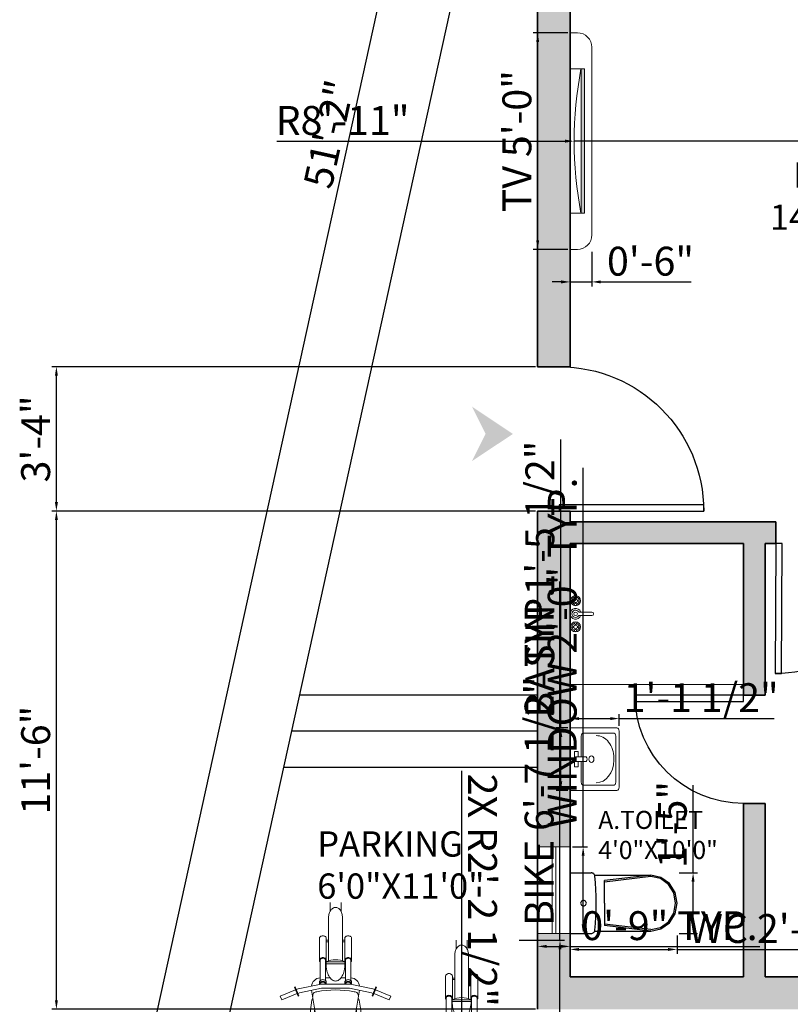
# Model space of a CAD drawing. Units: inches. Extents: x 2642 to 4124, y 1227 to 1973.
# Tile 2 of 7: x 3343 to 3556, y 1372 to 1645. Entities that reach past the tile are written whole.
import ezdxf

# ---------------------------------------------------------------- set-up
doc = ezdxf.new("R2010")
doc.units = ezdxf.units.IN
for name, color, linetype, lineweight in [('A-ANNO-DIMS', 2, 'Continuous', 18), ('A-ANNO-SYMB', 1, 'Continuous', 18), ('A-AREA-IDEN', 7, 'Continuous', 18), ('A-DOOR', 3, 'Continuous', 25), ('A-EQPM', 8, 'Continuous', 18), ('A-FLOR-STRS', 7, 'Continuous', 25), ('A-WALL', 7, 'Continuous', 35), ('A-WALL-PATT', 7, 'Continuous', 13), ('C-PRKG-VEHI', 8, 'Continuous', 18), ('C-PROP', 7, 'Continuous', 25), ('window', 4, 'Continuous', 18), ('Сантехника', 9, 'Continuous', 18)]:
    doc.layers.add(name, color=color, linetype=linetype, lineweight=lineweight)
doc.layers.add('SANTEH', color=7, linetype='Continuous')
doc.styles.get("Standard").update_dxf_attribs({"font": 'arial.ttf'})
doc.dimstyles.new('ISO-25', dxfattribs={"dimtxt": 8, "dimasz": 2.5, "dimexe": 1.25, "dimexo": 0.625, "dimtad": 1, "dimdec": 0, "dimlunit": 3, "dimtxsty": 'Standard', "dimcen": 2.5, "dimadec": 0, "dimazin": 0, "dimtfac": 1, "dimtdec": 0, "dimtmove": 0, "dimatfit": 3, "dimfxl": 1, "dimarcsym": 0})

# ---------------------------------------------------------------- blocks, each defined once
blk = doc.blocks.new('*D4')
at = {"layer": 'A-ANNO-DIMS', "color": 0, "lineweight": -2, "transparency": 16777216}
for p, q in [((3518.61, 1907.92), (3498.8, 1912.28)), ((3368.56, 1314.45), (3499.49, 1909.57)), ((3386.61, 1307.92), (3366.8, 1312.28))]:
    blk.add_line(p, q, dxfattribs=at)
at = {"layer": 'A-ANNO-DIMS', "color": 0, "transparency": 16777216}
for points in [[(3499.08, 1909.65), (3499.89, 1909.48), (3500.02, 1912.01)], [(3368.15, 1314.54), (3368.97, 1314.36), (3368.02, 1312.01)]]:
    blk.add_solid(points, dxfattribs=at)
at = {"layer": 'Defpoints', "color": 0, "transparency": 16777216}
for p in [(3500.02, 1912.01), (3519.22, 1907.78), (3387.22, 1307.78)]:
    blk.add_point(p, dxfattribs=at)
at = {"layer": 'A-ANNO-DIMS', "color": 0, "transparency": 16777216, "insert": (3429.42, 1613.02), "char_height": 8, "attachment_point": 5, "rotation": 77.5926}
blk.add_mtext('51\'-2"', dxfattribs=at)
blk = doc.blocks.new('*U11')
for p, q in [((0, 0), (0, -6)), ((30, 0), (30, -6))]:
    blk.add_line(p, q)
blk.add_lwpolyline([(0, 0), (0, 30), (1.75, 30), (1.75, 0)], close=True)
blk.add_arc((0, 0), 30, 0, 90)
blk = doc.blocks.new('*U10')
for p, q in [((0, 0), (0, -6)), ((36, 0), (36, -6))]:
    blk.add_line(p, q)
blk.add_lwpolyline([(0, 0), (0, 36), (1.75, 36), (1.75, 0)], close=True)
blk.add_arc((0, 0), 36, 0, 90)
blk = doc.blocks.new('*U13')
for p, q in [((0, 0), (0, -6)), ((40, 0), (40, -6))]:
    blk.add_line(p, q)
blk.add_lwpolyline([(0, 0), (0, 40), (1.75, 40), (1.75, 0)], close=True)
blk.add_arc((0, 0), 40, 0, 90)
blk = doc.blocks.new('TV 1')
at = {"transparency": 33554687}
h = blk.add_hatch(color=256, dxfattribs=at)
h.dxf.hatch_style = 1
h.paths.add_polyline_path([(3528.27, 1618.89), (3528.27, 1617.89), (3568.27, 1617.89), (3568.27, 1618.89)])
for p, q in [((3574.27, 1620.89), (3522.27, 1620.89)), ((3528.27, 1614.89), (3528.27, 1618.89)), ((3528.27, 1618.89), (3568.27, 1618.89)), ((3528.27, 1617.89), (3568.27, 1617.89)), ((3568.27, 1614.89), (3568.27, 1618.89)), ((3518.27, 1614.89), (3518.27, 1616.89)), ((3578.27, 1614.89), (3578.27, 1616.89)), ((3518.27, 1614.89), (3578.27, 1614.89))]:
    blk.add_line(p, q)
for centre, radius, start, end in [((3522.27, 1616.89), 4, 90, 180), ((3574.27, 1616.89), 4, 0, 90), ((3548.27, 1722.92), 106.92, 259.2189, 280.7811)]:
    blk.add_arc(centre, radius, start, end)
blk = doc.blocks.new('Rac7')
at = {"color": 0}
for p, q in [((-39473.6, -23808.4), (-38988.3, -23808.4)), ((-39500.6, -24232.1), (-39500.6, -23829.6)), ((-39456.5, -23859.1), (-39456.5, -24114.9)), ((-39032.4, -23838), (-39429.6, -23838)), ((-39221.1, -23854.9), (-39240.8, -23854.9)), ((-39005.4, -24114.9), (-39005.4, -23859.1)), ((-39005.4, -23859.1), (-39005.4, -23859.1)), ((-38961.3, -23829.6), (-38961.3, -24232.1)), ((-39429.6, -24136.1), (-39252.5, -24136.1)), ((-39252.5, -24185.9), (-39252.5, -24093.6)), ((-39209.4, -24185.9), (-39209.4, -24093.6)), ((-39209.4, -24136.1), (-39032.4, -24136.1)), ((-38961.3, -24232.1), (-39500.6, -24232.1)), ((-39297, -24164), (-39252.5, -24164)), ((-39297, -24193.5), (-39297, -24164)), ((-39164.9, -24193.5), (-39297, -24193.5)), ((-39252.5, -24185.9), (-39209.4, -24185.9)), ((-39209.4, -24164), (-39164.9, -24164)), ((-39164.9, -24164), (-39164.9, -24193.5))]:
    blk.add_line(p, q, dxfattribs=at)
at = {"color": 0, "extrusion": (0, 0, -1)}
for centre, major_axis, start_param, end_param in [((-39473.6, -23829.6), (-27, 0), 0, 1.570796), ((-38988.3, -23829.6), (-27, 0), 1.570796, 3.141593), ((-39429.6, -23859.1), (-27, 0), 0, 1.570796), ((-39240.8, -24007.4), (-194.1, 0), 0, 1.570796), ((-39221.1, -24007.4), (-194.1, 0), 1.570796, 3.141593), ((-39032.4, -23859.1), (-27, 0), 1.570796, 3.141593), ((-39429.6, -24114.9), (-27, 0), -1.570796, 0), ((-39231, -24104), (-25.3, 0), 0.552816, 2.588777), ((-39032.4, -24114.9), (-27, 0), -3.141593, -1.570796)]:
    blk.add_ellipse(centre, major_axis=major_axis, ratio=0.785714, start_param=start_param, end_param=end_param, dxfattribs=at)
blk.add_ellipse((-39231, -24048), major_axis=(-27.9, 0), ratio=0.785714, dxfattribs=at)
blk = doc.blocks.new('Faucet - Bathroom top')
for p, q in [((-4.107, 0.125), (-4.375, 0.125)), ((-3.75, 0.4788), (-3.75, 0.75)), ((-3.5, 0.482), (-3.5, 0.75)), ((-3.1461, 0.125), (-2.875, 0.125)), ((3.143, 0.125), (2.875, 0.125)), ((3.5, 0.4788), (3.5, 0.75)), ((3.75, 0.482), (3.75, 0.75)), ((4.1039, 0.125), (4.375, 0.125)), ((-4.1039, -0.125), (-4.375, -0.125)), ((-3.75, -0.4821), (-3.75, -0.75)), ((-3.5, -0.4789), (-3.5, -0.75)), ((-3.143, -0.125), (-2.875, -0.125)), ((-0.5, -0.8639), (-0.5, -4.5)), ((0.5, -4.5), (0.5, -0.8631)), ((3.1461, -0.125), (2.875, -0.125)), ((3.5, -0.4821), (3.5, -0.75)), ((3.75, -0.4789), (3.75, -0.75)), ((4.107, -0.125), (4.375, -0.125))]:
    blk.add_line(p, q)
for centre, radius in [((-3.625, 0), 1.375), ((-4.625, 0), 0.2795), ((-3.625, 0), 0.5), ((-3.625, 1), 0.2795), ((-2.625, 0), 0.2795), ((0, 0), 0.5), ((3.625, 0), 1.375), ((2.625, 0), 0.2795), ((3.625, 0), 0.5), ((3.625, 1), 0.2795), ((4.625, 0), 0.2795), ((-3.625, -1), 0.2795), ((3.625, -1), 0.2795)]:
    blk.add_circle(centre, radius)
for centre, radius, start, end in [((-3.625, 0), 1, 105.2407, 164.2093), ((-3.625, 0), 1, 16.44125, 74.07887), ((0, 0), 1.5, 289.6514, 250.3603), ((0, 0), 1, 300.3431, 239.7554), ((3.625, 0), 1, 106.12, 164.0884), ((3.625, 0), 1, 16.23422, 73.90469), ((-3.625, 0), 1, 196.2342, 253.9047), ((-3.625, 0), 1, 286.12, 344.0884), ((3.625, 0), 1, 196.4413, 254.0789), ((3.625, 0), 1, 285.2407, 344.2093), ((0, -4.5), 0.5, 180, 0)]:
    blk.add_arc(centre, radius, start, end)
blk = doc.blocks.new('WC 2 Symb_109')
at = {"layer": 'SANTEH'}
for p, q in [((0, 0), (0, 380)), ((0, 380), (132.4, 380)), ((153.6, 364.9), (506.8, 364.9)), ((506.3, 364.9), (215.7, 330.9)), ((506.3, 356), (215.7, 322)), ((215.7, 190), (215.7, 330.9)), ((215.7, 190), (215.7, 49.1)), ((153.8, 15.1), (506.8, 15.1)), ((506.3, 24), (215.7, 58)), ((506.3, 15.1), (215.7, 49.1)), ((0, 0), (132.4, 0))]:
    blk.add_line(p, q, dxfattribs=at)
for points in [[(154.6, 360.1), (153.9, 364.1), (152.3, 367.9), (150.2, 371.3), (147.4, 374.3), (144.1, 376.7), (140.5, 378.5), (136.5, 379.6), (132.4, 380)], [(154.6, 19.7), (158.6, 62.1), (161.4, 104.7), (163.1, 147.3), (163.7, 189.9), (163.1, 232.5), (161.4, 275.1), (158.6, 317.7), (154.6, 360.1)], [(506.3, 24), (565.5, 36.6), (615.7, 72.6), (649.2, 126.5), (661, 190), (649.2, 253.5), (615.7, 307.4), (565.5, 343.4), (506.3, 356)], [(506.8, 15.1), (569.2, 28.4), (622.2, 66.3), (657.6, 123.1), (670, 190), (657.6, 256.9), (622.2, 313.7), (569.2, 351.6), (506.8, 364.9)], [(132.4, 0), (136.5, 0.4), (140.4, 1.5), (144.1, 3.2), (147.3, 5.6), (150.1, 8.6), (152.3, 12), (153.8, 15.7), (154.6, 19.7)]]:
    blk.add_lwpolyline(points, dxfattribs=at)
blk.add_lwpolyline([(83.6, 208.5), (70.4, 203.1), (64.9, 190), (70.4, 176.9), (83.6, 171.5), (96.8, 176.9), (102.2, 190), (96.8, 203.1)], close=True, dxfattribs=at)
blk = doc.blocks.new('BIKE')
for p, q in [((34846.04, 15170.34), (34846.04, 15168.87)), ((34847.86, 15170.34), (34847.86, 15168.87)), ((34845.81, 15167.86), (34845.81, 15160.7)), ((34845.81, 15167.86), (34845.81, 15160.7)), ((34848.09, 15167.86), (34848.09, 15160.7)), ((34844.29, 15164.4), (34844.29, 15160.81)), ((34845.43, 15164.4), (34845.43, 15160.81)), ((34845.43, 15164.1), (34845.81, 15164.1)), ((34845.43, 15163.85), (34845.81, 15163.85)), ((34848.47, 15164.1), (34848.09, 15164.1)), ((34848.47, 15163.85), (34848.09, 15163.85)), ((34848.47, 15164.4), (34848.47, 15160.81)), ((34849.61, 15164.4), (34849.61, 15160.81)), ((34844.41, 15160.81), (34844.41, 15157.43)), ((34845.32, 15160.81), (34845.32, 15157.43)), ((34848.51, 15160.53), (34845.39, 15160.53)), ((34845.39, 15160.23), (34845.39, 15160.53)), ((34845.39, 15160.23), (34845.39, 15160.53)), ((34848.51, 15160.23), (34845.39, 15160.23)), ((34848.51, 15160.23), (34848.51, 15160.53)), ((34848.58, 15160.81), (34848.58, 15157.43)), ((34849.5, 15160.81), (34849.5, 15157.43)), ((34840.8, 15156.11), (34844.56, 15156.88)), ((34844.29, 15156.87), (34844.29, 15157.17)), ((34844.41, 15156.87), (34844.41, 15156.85)), ((34844.56, 15156.88), (34846.95, 15156.88)), ((34845.32, 15157.92), (34846.04, 15157.92)), ((34845.43, 15156.87), (34845.43, 15157.17)), ((34849.34, 15156.88), (34846.95, 15156.88)), ((34848.58, 15157.92), (34847.87, 15157.92)), ((34848.47, 15156.87), (34848.47, 15157.17)), ((34853.1, 15156.11), (34849.34, 15156.88)), ((34849.5, 15156.87), (34849.5, 15156.85)), ((34849.61, 15156.87), (34849.61, 15157.17)), ((34837.84, 15154.89), (34840.37, 15155.93)), ((34838.1, 15154.26), (34840.63, 15155.3)), ((34840.19, 15156.35), (34840.3, 15156.39)), ((34840.19, 15156.35), (34840.8, 15154.88)), ((34840.3, 15156.39), (34840.9, 15154.92)), ((34840.47, 15155.97), (34840.8, 15156.11)), ((34840.73, 15155.34), (34841, 15155.45)), ((34841, 15155.45), (34844.63, 15156.2)), ((34844.86, 15144.72), (34843.01, 15155.87)), ((34844.63, 15156.2), (34846.95, 15156.2)), ((34849.27, 15156.2), (34846.95, 15156.2)), ((34849.05, 15144.72), (34850.89, 15155.87)), ((34852.9, 15155.45), (34849.27, 15156.2)), ((34853.17, 15155.34), (34852.9, 15155.45)), ((34853.6, 15156.39), (34853, 15154.92)), ((34853.71, 15156.35), (34853.1, 15154.88)), ((34853.43, 15155.97), (34853.1, 15156.11)), ((34855.81, 15154.26), (34853.28, 15155.3)), ((34856.07, 15154.89), (34853.54, 15155.93)), ((34853.71, 15156.35), (34853.6, 15156.39)), ((34837.84, 15154.89), (34838.1, 15154.26)), ((34840.8, 15154.88), (34840.9, 15154.92)), ((34842.8, 15152.59), (34843.06, 15154.2)), ((34843.06, 15154.2), (34843.22, 15154.58)), ((34850.84, 15154.2), (34850.68, 15154.58)), ((34851.1, 15152.59), (34850.84, 15154.2)), ((34853.1, 15154.88), (34853, 15154.92)), ((34856.07, 15154.89), (34855.81, 15154.26)), ((34842.7, 15150.31), (34842.8, 15152.59)), ((34843.33, 15151.09), (34843.52, 15152.8)), ((34850.57, 15151.09), (34850.38, 15152.8)), ((34851.2, 15150.31), (34851.1, 15152.59)), ((34840.97, 15150.31), (34843.3, 15150.31)), ((34840.97, 15149.81), (34840.97, 15150.31)), ((34843.23, 15147.75), (34843.33, 15151.09)), ((34850.67, 15147.75), (34850.57, 15151.09)), ((34852.93, 15150.31), (34850.6, 15150.31)), ((34852.93, 15149.81), (34852.93, 15150.31)), ((34843.29, 15149.81), (34840.97, 15149.81)), ((34842.7, 15144.87), (34842.7, 15149.81)), ((34850.61, 15149.81), (34852.93, 15149.81)), ((34851.2, 15144.87), (34851.2, 15149.81)), ((34843.23, 15144.15), (34843.23, 15147.75)), ((34850.67, 15144.15), (34850.67, 15147.75)), ((34842.7, 15144.87), (34842.25, 15142.19)), ((34842.7, 15144.87), (34843.23, 15144.87)), ((34847.85, 15144.64), (34846.06, 15144.64)), ((34851.2, 15144.87), (34850.67, 15144.87)), ((34851.2, 15144.87), (34851.65, 15142.19)), ((34842.25, 15142.19), (34844.07, 15142.19)), ((34842.25, 15137.82), (34842.25, 15142.19)), ((34844.46, 15143.56), (34843.6, 15128.2)), ((34843.85, 15143.46), (34844.07, 15142.19)), ((34843.91, 15143.46), (34844.46, 15143.46)), ((34844.07, 15137.82), (34844.07, 15142.19)), ((34849.44, 15143.56), (34850.3, 15128.2)), ((34849.99, 15143.46), (34849.44, 15143.46)), ((34850.05, 15143.46), (34849.83, 15142.19)), ((34851.65, 15142.19), (34849.83, 15142.19)), ((34849.83, 15137.82), (34849.83, 15142.19)), ((34851.65, 15137.82), (34851.65, 15142.19)), ((34841.79, 15137.82), (34844.14, 15137.82)), ((34841.79, 15137.33), (34841.79, 15137.82)), ((34844.11, 15137.33), (34841.79, 15137.33)), ((34842.25, 15127.57), (34842.25, 15137.33)), ((34844.07, 15136.55), (34844.07, 15137.33)), ((34852.11, 15137.82), (34849.76, 15137.82)), ((34849.79, 15137.33), (34852.11, 15137.33)), ((34849.83, 15136.55), (34849.83, 15137.33)), ((34851.65, 15127.57), (34851.65, 15137.33)), ((34852.11, 15137.33), (34852.11, 15137.82)), ((34842.25, 15127.57), (34843.75, 15127.57)), ((34842.25, 15127.57), (34842.48, 15126.27)), ((34851.65, 15127.57), (34850.15, 15127.57)), ((34851.65, 15127.57), (34851.43, 15126.27)), ((34842.48, 15126.27), (34843.84, 15126.27)), ((34844.02, 15127.25), (34843.84, 15126.27)), ((34849.16, 15126.99), (34844.74, 15126.99)), ((34845.47, 15126.99), (34845.47, 15126.88)), ((34845.81, 15126.99), (34845.81, 15126.88)), ((34845.81, 15126.29), (34845.81, 15124.03)), ((34847.75, 15126.54), (34846.15, 15126.54)), ((34847.75, 15126.2), (34846.15, 15126.2)), ((34848.09, 15126.99), (34848.09, 15126.88)), ((34848.09, 15126.29), (34848.09, 15124.03)), ((34848.43, 15126.99), (34848.43, 15126.88)), ((34849.89, 15127.25), (34850.06, 15126.27)), ((34851.43, 15126.27), (34850.06, 15126.27)), ((34846.29, 15123.82), (34846.29, 15124.66)), ((34846.29, 15124.66), (34847.61, 15124.66)), ((34846.29, 15124.55), (34847.61, 15124.55)), ((34847.61, 15124.66), (34847.61, 15123.82)), ((34847.61, 15123.82), (34846.29, 15123.82))]:
    blk.add_line(p, q)
for points in [[(34845.81, 15167.86, -0.068977), (34845.9, 15168.53, -0.081012), (34846.15, 15169.05, -0.107014), (34846.54, 15169.42, -0.137239), (34846.95, 15169.53, -0.137239), (34847.36, 15169.42, -0.107014), (34847.76, 15169.05, -0.081012), (34848, 15168.53, -0.068977), (34848.09, 15167.86, -0.068977)], [(34845.43, 15164.4, 0.125099), (34845.39, 15164.56, 0.105827), (34845.27, 15164.71, 0.086577), (34845.09, 15164.8, 0.0766), (34844.86, 15164.84, 0.0766), (34844.64, 15164.8, 0.086577), (34844.46, 15164.71, 0.105827), (34844.33, 15164.56, 0.125099), (34844.29, 15164.4, 0.125099)], [(34848.47, 15164.4, -0.125099), (34848.51, 15164.56, -0.105827), (34848.64, 15164.71, -0.086577), (34848.82, 15164.8, -0.0766), (34849.04, 15164.84, -0.0766), (34849.26, 15164.8, -0.086577), (34849.44, 15164.71, -0.105827), (34849.57, 15164.56, -0.125099), (34849.61, 15164.4, -0.125099)], [(34845.32, 15160.55, 0.067261), (34845.39, 15160.65, 0.125099), (34845.43, 15160.81, 0.125099), (34845.39, 15160.97, 0.105827), (34845.27, 15161.12, 0.086577), (34845.09, 15161.21, 0.0766), (34844.86, 15161.25, 0.0766), (34844.64, 15161.21, 0.086577), (34844.46, 15161.12, 0.105827), (34844.33, 15160.97, 0.125099), (34844.29, 15160.81, 0.125099)], [(34844.29, 15160.81, 0.125099), (34844.33, 15160.65, 0.067261), (34844.41, 15160.55, 0.086577)], [(34845.32, 15160.81, 0.125099), (34845.29, 15160.92, 0.105827), (34845.2, 15161.03, 0.086577), (34845.05, 15161.1, 0.0766), (34844.86, 15161.13, 0.0766), (34844.67, 15161.1, 0.086577), (34844.53, 15161.03, 0.105827), (34844.43, 15160.92, 0.125099), (34844.41, 15160.81, 0.125099)], [(34846.95, 15157.37, -0.163989), (34846.41, 15157.55, -0.105862), (34845.85, 15158.21, -0.069323), (34845.52, 15159.08, -0.055531), (34845.39, 15160.23, -0.055531)], [(34848.51, 15160.23, -0.055531), (34848.38, 15159.08, -0.069323), (34848.06, 15158.21, -0.105862), (34847.49, 15157.55, -0.163989), (34846.95, 15157.37, -0.163989)], [(34848.58, 15160.55, -0.067261), (34848.51, 15160.65, -0.125099), (34848.47, 15160.81, -0.125099), (34848.51, 15160.97, -0.105827), (34848.64, 15161.12, -0.086577), (34848.82, 15161.21, -0.0766), (34849.04, 15161.25, -0.0766), (34849.26, 15161.21, -0.086577), (34849.44, 15161.12, -0.105827), (34849.57, 15160.97, -0.125099), (34849.61, 15160.81, -0.125099)], [(34848.58, 15160.81, -0.125099), (34848.61, 15160.92, -0.105827), (34848.71, 15161.03, -0.086577), (34848.85, 15161.1, -0.0766), (34849.04, 15161.13, -0.0766), (34849.23, 15161.1, -0.086577), (34849.37, 15161.03, -0.105827), (34849.47, 15160.92, -0.125099), (34849.5, 15160.81, -0.125099)], [(34849.61, 15160.81, -0.125099), (34849.57, 15160.65, -0.067261), (34849.5, 15160.55, -0.086577)], [(34845.43, 15157.17, 0.125099), (34845.39, 15157.33, 0.105827), (34845.27, 15157.48, 0.086577), (34845.09, 15157.57, 0.0766), (34844.86, 15157.6, 0.0766), (34844.64, 15157.57, 0.086577), (34844.46, 15157.48, 0.105827), (34844.33, 15157.33, 0.125099), (34844.29, 15157.17, 0.125099)], [(34845.43, 15156.88, 0.117252), (34845.39, 15157.03, 0.105827), (34845.27, 15157.18, 0.086577), (34845.09, 15157.27, 0.0766), (34844.86, 15157.31, 0.0766), (34844.64, 15157.27, 0.086577), (34844.46, 15157.18, 0.105827), (34844.33, 15157.03, 0.125099), (34844.29, 15156.87, 0.125099)], [(34844.29, 15156.87, 0.032819), (34844.3, 15156.83, 0.067261)], [(34845.32, 15156.88, 0.113202), (34845.29, 15156.98, 0.105827), (34845.2, 15157.09, 0.086577), (34845.05, 15157.16, 0.0766), (34844.86, 15157.19, 0.0766), (34844.67, 15157.16, 0.086577), (34844.53, 15157.09, 0.105827), (34844.43, 15156.98, 0.125099), (34844.41, 15156.87, 0.125099)], [(34848.47, 15157.17, -0.125099), (34848.51, 15157.33, -0.105827), (34848.64, 15157.48, -0.086577), (34848.82, 15157.57, -0.0766), (34849.04, 15157.6, -0.0766), (34849.26, 15157.57, -0.086577), (34849.44, 15157.48, -0.105827), (34849.57, 15157.33, -0.125099), (34849.61, 15157.17, -0.125099)], [(34848.47, 15156.88, -0.117252), (34848.51, 15157.03, -0.105827), (34848.64, 15157.18, -0.086577), (34848.82, 15157.27, -0.0766), (34849.04, 15157.31, -0.0766), (34849.26, 15157.27, -0.086577), (34849.44, 15157.18, -0.105827), (34849.57, 15157.03, -0.125099), (34849.61, 15156.87, -0.125099)], [(34848.58, 15156.88, -0.113202), (34848.61, 15156.98, -0.105827), (34848.71, 15157.09, -0.086577), (34848.85, 15157.16, -0.0766), (34849.04, 15157.19, -0.0766), (34849.23, 15157.16, -0.086577), (34849.37, 15157.09, -0.105827), (34849.47, 15156.98, -0.125099), (34849.5, 15156.87, -0.125099)], [(34849.61, 15156.87, -0.032819), (34849.61, 15156.83, -0.067261)]]:
    blk.add_lwpolyline(points, format="xyb")
for centre, radius, start, end in [((34846.95, 15157.24), 3.64, 64.5882, 115.4118), ((34844.55, 15156.32), 1.59, 95.2207, 171.678), ((34849.35, 15156.32), 1.59, 8.322, 84.7793), ((34843.86, 15154.92), 0.684, 90, 189.3898), ((34846.95, 15140.12), 15.79, 78.7129, 101.2871), ((34850.04, 15154.92), 0.684, 350.6102, 90), ((34843.91, 15144.15), 0.684, 180, 270), ((34846, 15143), 1.64, 88.1125, 159.9264), ((34845.53, 15144.83), 0.684, 189.3898, 226.4877), ((34847.9, 15143), 1.64, 20.0736, 91.8875), ((34848.37, 15144.83), 0.684, 313.5123, 350.6102), ((34849.99, 15144.15), 0.684, 270, 0), ((34844.74, 15128.13), 1.14, 176.7865, 270), ((34849.16, 15128.13), 1.14, 270, 3.2135), ((34846.15, 15126.88), 0.684, 180, 270), ((34846.15, 15126.88), 0.342, 180, 270), ((34847.75, 15126.88), 0.684, 270, 0), ((34847.75, 15126.88), 0.342, 270, 0), ((34846.95, 15124.03), 1.14, 180, 0)]:
    blk.add_arc(centre, radius, start, end)
blk = doc.blocks.new('WIN-24IN')
for p, q in [((0, 24), (9, 24)), ((4, 24), (4, 0)), ((5, 24), (5, 0)), ((0, 0), (9, 0))]:
    blk.add_line(p, q)
blk = doc.blocks.new('*D42')
at = {"layer": 'A-ANNO-DIMS', "color": 0, "lineweight": -2, "transparency": 16777216}
for p, q in [((3498.82, 1415.78), (3498.82, 1520.77)), ((3495.85, 1415.78), (3500.07, 1415.78)), ((3498.82, 1394.28), (3498.82, 1413.28)), ((3495.85, 1391.78), (3500.07, 1391.78))]:
    blk.add_line(p, q, dxfattribs=at)
at = {"layer": 'A-ANNO-DIMS', "color": 0, "transparency": 16777216}
for points in [[(3498.41, 1413.28), (3499.24, 1413.28), (3498.82, 1415.78)], [(3498.41, 1394.28), (3499.24, 1394.28), (3498.82, 1391.78)]]:
    blk.add_solid(points, dxfattribs=at)
at = {"layer": 'Defpoints', "color": 0, "transparency": 16777216}
for p in [(3495.22, 1415.78), (3498.82, 1415.78), (3495.22, 1391.78)]:
    blk.add_point(p, dxfattribs=at)
at = {"layer": 'A-ANNO-DIMS', "color": 0, "transparency": 16777216, "insert": (3494.06, 1469.52), "char_height": 8, "attachment_point": 5, "rotation": 90}
blk.add_mtext('WINDOW 2\'-0" TYP.', dxfattribs=at)
blk = doc.blocks.new('*D43')
at = {"layer": 'A-ANNO-DIMS', "color": 0, "lineweight": -2, "transparency": 16777216}
for p, q in [((3486.22, 1391.16), (3486.22, 1386.93)), ((3495.22, 1391.16), (3495.22, 1386.93)), ((3488.72, 1388.18), (3492.72, 1388.18)), ((3495.22, 1388.18), (3547.74, 1388.18))]:
    blk.add_line(p, q, dxfattribs=at)
at = {"layer": 'A-ANNO-DIMS', "color": 0, "transparency": 16777216}
for points in [[(3488.72, 1388.6), (3488.72, 1387.77), (3486.22, 1388.18)], [(3492.72, 1388.6), (3492.72, 1387.77), (3495.22, 1388.18)]]:
    blk.add_solid(points, dxfattribs=at)
at = {"layer": 'Defpoints', "color": 0, "transparency": 16777216}
for p in [(3486.22, 1391.78), (3495.22, 1391.78), (3495.22, 1388.18)]:
    blk.add_point(p, dxfattribs=at)
at = {"layer": 'A-ANNO-DIMS', "color": 0, "transparency": 16777216, "insert": (3522.73, 1392.89), "char_height": 8, "attachment_point": 5}
blk.add_mtext('0\'-9" TYP.', dxfattribs=at)
blk = doc.blocks.new('*D48')
at = {"layer": 'A-ANNO-DIMS', "color": 0, "lineweight": -2, "transparency": 16777216}
for p, q in [((3492.41, 1389.89), (3492.41, 1489.27)), ((3481.09, 1389.89), (3493.66, 1389.89)), ((3492.41, 1312.73), (3492.41, 1387.39)), ((3481.09, 1310.23), (3493.66, 1310.23))]:
    blk.add_line(p, q, dxfattribs=at)
at = {"layer": 'A-ANNO-DIMS', "color": 0, "transparency": 16777216}
for points in [[(3492, 1387.39), (3492.83, 1387.39), (3492.41, 1389.89)], [(3492, 1312.73), (3492.83, 1312.73), (3492.41, 1310.23)]]:
    blk.add_solid(points, dxfattribs=at)
at = {"layer": 'Defpoints', "color": 0, "transparency": 16777216}
for p in [(3480.46, 1389.89), (3492.41, 1389.89), (3480.46, 1310.23)]:
    blk.add_point(p, dxfattribs=at)
at = {"layer": 'A-ANNO-DIMS', "color": 0, "transparency": 16777216, "insert": (3487.65, 1440.83), "char_height": 8, "attachment_point": 5, "rotation": 90}
blk.add_mtext('BIKE 6\'-7 1/2" TYP.', dxfattribs=at)
blk = doc.blocks.new('*D50')
at = {"layer": 'A-ANNO-DIMS', "color": 0, "lineweight": -2, "transparency": 16777216}
for p, q in [((3494.6, 1641.28), (3484.97, 1641.28)), ((3486.22, 1638.78), (3486.22, 1583.78)), ((3494.6, 1581.28), (3484.97, 1581.28))]:
    blk.add_line(p, q, dxfattribs=at)
at = {"layer": 'A-ANNO-DIMS', "color": 0, "transparency": 16777216}
for points in [[(3485.81, 1638.78), (3486.64, 1638.78), (3486.22, 1641.28)], [(3485.81, 1583.78), (3486.64, 1583.78), (3486.22, 1581.28)]]:
    blk.add_solid(points, dxfattribs=at)
at = {"layer": 'Defpoints', "color": 0, "transparency": 16777216}
for p in [(3495.22, 1641.28), (3486.22, 1581.28), (3495.22, 1581.28)]:
    blk.add_point(p, dxfattribs=at)
at = {"layer": 'A-ANNO-DIMS', "color": 0, "transparency": 16777216, "insert": (3481.51, 1611.28), "char_height": 8, "attachment_point": 5, "rotation": 90}
blk.add_mtext('TV 5\'-0"', dxfattribs=at)
blk = doc.blocks.new('*D51')
at = {"layer": 'A-ANNO-DIMS', "color": 0, "lineweight": -2, "transparency": 16777216}
for p, q in [((3495.22, 1580.66), (3495.22, 1571.03)), ((3501.22, 1580.66), (3501.22, 1571.03)), ((3492.72, 1572.28), (3490.22, 1572.28)), ((3495.22, 1572.28), (3501.22, 1572.28)), ((3503.72, 1572.28), (3528.74, 1572.28))]:
    blk.add_line(p, q, dxfattribs=at)
at = {"layer": 'A-ANNO-DIMS', "color": 0, "transparency": 16777216}
for points in [[(3492.72, 1572.7), (3492.72, 1571.87), (3495.22, 1572.28)], [(3503.72, 1572.7), (3503.72, 1571.87), (3501.22, 1572.28)]]:
    blk.add_solid(points, dxfattribs=at)
at = {"layer": 'Defpoints', "color": 0, "transparency": 16777216}
for p in [(3495.22, 1581.28), (3501.22, 1581.28), (3501.22, 1572.28)]:
    blk.add_point(p, dxfattribs=at)
at = {"layer": 'A-ANNO-DIMS', "color": 0, "transparency": 16777216, "insert": (3517.48, 1576.99), "char_height": 8, "attachment_point": 5}
blk.add_mtext('0\'-6"', dxfattribs=at)
blk = doc.blocks.new('*D62')
at = {"layer": 'A-ANNO-DIMS', "color": 0, "lineweight": -2, "transparency": 16777216}
for p, q in [((3492.63, 1448.7), (3492.63, 1528.65)), ((3494.6, 1448.7), (3491.38, 1448.7)), ((3492.63, 1433.91), (3492.63, 1446.2)), ((3494.6, 1431.41), (3491.38, 1431.41))]:
    blk.add_line(p, q, dxfattribs=at)
at = {"layer": 'A-ANNO-DIMS', "color": 0, "transparency": 16777216}
for points in [[(3492.21, 1446.2), (3493.04, 1446.2), (3492.63, 1448.7)], [(3492.21, 1433.91), (3493.04, 1433.91), (3492.63, 1431.41)]]:
    blk.add_solid(points, dxfattribs=at)
at = {"layer": 'Defpoints', "color": 0, "transparency": 16777216}
for p in [(3492.63, 1448.7), (3495.22, 1448.7), (3495.22, 1431.41)]:
    blk.add_point(p, dxfattribs=at)
at = {"layer": 'A-ANNO-DIMS', "color": 0, "transparency": 16777216, "insert": (3487.87, 1489.93), "char_height": 8, "attachment_point": 5, "rotation": 90}
blk.add_mtext('BASIN 1\'-5 1/2"', dxfattribs=at)
blk = doc.blocks.new('*D63')
at = {"layer": 'A-ANNO-DIMS', "color": 0, "lineweight": -2, "transparency": 16777216}
for p, q in [((3495.22, 1449.33), (3495.22, 1452.55)), ((3497.72, 1451.3), (3506.31, 1451.3)), ((3508.81, 1449.33), (3508.81, 1452.55)), ((3508.81, 1451.3), (3551.71, 1451.3))]:
    blk.add_line(p, q, dxfattribs=at)
at = {"layer": 'A-ANNO-DIMS', "color": 0, "transparency": 16777216}
for points in [[(3497.72, 1451.71), (3497.72, 1450.88), (3495.22, 1451.3)], [(3506.31, 1451.71), (3506.31, 1450.88), (3508.81, 1451.3)]]:
    blk.add_solid(points, dxfattribs=at)
at = {"layer": 'Defpoints', "color": 0, "transparency": 16777216}
for p in [(3508.81, 1451.3), (3495.22, 1448.7), (3508.81, 1448.7)]:
    blk.add_point(p, dxfattribs=at)
at = {"layer": 'A-ANNO-DIMS', "color": 0, "transparency": 16777216, "insert": (3531.51, 1456.06), "char_height": 8, "attachment_point": 5}
blk.add_mtext('1\'-1 1/2"', dxfattribs=at)
blk = doc.blocks.new('*D64')
at = {"layer": 'A-ANNO-DIMS', "color": 0, "lineweight": -2, "transparency": 16777216}
for p, q in [((3495.22, 1391.16), (3495.22, 1386.09)), ((3524.83, 1391.16), (3524.83, 1386.09)), ((3497.72, 1387.34), (3522.33, 1387.34)), ((3524.83, 1387.34), (3590.54, 1387.34))]:
    blk.add_line(p, q, dxfattribs=at)
at = {"layer": 'A-ANNO-DIMS', "color": 0, "transparency": 16777216}
for points in [[(3497.72, 1387.76), (3497.72, 1386.93), (3495.22, 1387.34)], [(3522.33, 1387.76), (3522.33, 1386.93), (3524.83, 1387.34)]]:
    blk.add_solid(points, dxfattribs=at)
at = {"layer": 'Defpoints', "color": 0, "transparency": 16777216}
for p in [(3495.22, 1391.78), (3524.83, 1391.78), (3524.83, 1387.34)]:
    blk.add_point(p, dxfattribs=at)
at = {"layer": 'A-ANNO-DIMS', "color": 0, "transparency": 16777216, "insert": (3558.93, 1392.1), "char_height": 8, "attachment_point": 5}
blk.add_mtext('WC 2\'-5 1/2"', dxfattribs=at)
blk = doc.blocks.new('*D65')
at = {"layer": 'A-ANNO-DIMS', "color": 0, "lineweight": -2, "transparency": 16777216}
for p, q in [((3529.27, 1408.58), (3529.27, 1432.84)), ((3525.45, 1408.58), (3530.52, 1408.58)), ((3529.27, 1394.28), (3529.27, 1406.08)), ((3525.45, 1391.78), (3530.52, 1391.78))]:
    blk.add_line(p, q, dxfattribs=at)
at = {"layer": 'A-ANNO-DIMS', "color": 0, "transparency": 16777216}
for points in [[(3528.85, 1406.08), (3529.69, 1406.08), (3529.27, 1408.58)], [(3528.85, 1394.28), (3529.69, 1394.28), (3529.27, 1391.78)]]:
    blk.add_solid(points, dxfattribs=at)
at = {"layer": 'Defpoints', "color": 0, "transparency": 16777216}
for p in [(3524.83, 1408.58), (3529.27, 1408.58), (3524.83, 1391.78)]:
    blk.add_point(p, dxfattribs=at)
at = {"layer": 'A-ANNO-DIMS', "color": 0, "transparency": 16777216, "insert": (3524.56, 1421.96), "char_height": 8, "attachment_point": 5, "rotation": 90}
blk.add_mtext('1\'-5"', dxfattribs=at)
blk = doc.blocks.new('*D71')
at = {"layer": 'A-ANNO-DIMS', "color": 0, "lineweight": -2, "transparency": 16777216}
for p, q in [((3485.6, 1548.78), (3351.67, 1548.78)), ((3352.92, 1511.28), (3352.92, 1546.28)), ((3485.6, 1508.78), (3351.67, 1508.78))]:
    blk.add_line(p, q, dxfattribs=at)
at = {"layer": 'A-ANNO-DIMS', "color": 0, "transparency": 16777216}
for points in [[(3352.51, 1546.28), (3353.34, 1546.28), (3352.92, 1548.78)], [(3352.51, 1511.28), (3353.34, 1511.28), (3352.92, 1508.78)]]:
    blk.add_solid(points, dxfattribs=at)
at = {"layer": 'Defpoints', "color": 0, "transparency": 16777216}
for p in [(3352.92, 1548.78), (3486.22, 1548.78), (3486.22, 1508.78)]:
    blk.add_point(p, dxfattribs=at)
at = {"layer": 'A-ANNO-DIMS', "color": 0, "transparency": 16777216, "insert": (3348.21, 1528.78), "char_height": 8, "attachment_point": 5, "rotation": 90}
blk.add_mtext('3\'-4"', dxfattribs=at)
blk = doc.blocks.new('*D72')
at = {"layer": 'A-ANNO-DIMS', "color": 0, "lineweight": -2, "transparency": 16777216}
for p, q in [((3485.6, 1508.78), (3351.67, 1508.78)), ((3352.92, 1373.28), (3352.92, 1506.28)), ((3485.6, 1370.78), (3351.67, 1370.78))]:
    blk.add_line(p, q, dxfattribs=at)
at = {"layer": 'A-ANNO-DIMS', "color": 0, "transparency": 16777216}
for points in [[(3352.51, 1506.28), (3353.34, 1506.28), (3352.92, 1508.78)], [(3352.51, 1373.28), (3353.34, 1373.28), (3352.92, 1370.78)]]:
    blk.add_solid(points, dxfattribs=at)
at = {"layer": 'Defpoints', "color": 0, "transparency": 16777216}
for p in [(3352.92, 1508.78), (3486.22, 1508.78), (3486.22, 1370.78)]:
    blk.add_point(p, dxfattribs=at)
at = {"layer": 'A-ANNO-DIMS', "color": 0, "transparency": 16777216, "insert": (3348.21, 1439.78), "char_height": 8, "attachment_point": 5, "rotation": 90}
blk.add_mtext('11\'-6"', dxfattribs=at)
blk = doc.blocks.new('*D83')
at = {"layer": 'A-ANNO-DIMS', "color": 0, "lineweight": -2, "transparency": 16777216}
for p, q in [((3413.99, 1611.28), (3493.83, 1611.28)), ((3603.25, 1611.28), (3496.33, 1611.28))]:
    blk.add_line(p, q, dxfattribs=at)
at = {"layer": 'A-ANNO-DIMS', "color": 0, "transparency": 16777216}
blk.add_solid([(3493.83, 1611.7), (3493.83, 1610.87), (3496.33, 1611.28)], dxfattribs=at)
at = {"layer": 'Defpoints', "color": 0, "transparency": 16777216}
for p in [(3496.33, 1611.28), (3603.25, 1611.28)]:
    blk.add_point(p, dxfattribs=at)
at = {"layer": 'A-ANNO-DIMS', "color": 0, "transparency": 16777216, "insert": (3432.18, 1615.99), "char_height": 8, "attachment_point": 5}
blk.add_mtext('R8\'-11"', dxfattribs=at)
blk = doc.blocks.new('*D84')
at = {"layer": 'A-ANNO-DIMS', "color": 0, "lineweight": -2, "transparency": 16777216}
for p, q in [((3465.16, 1436.8), (3465.16, 1368.17)), ((3465.16, 1339.16), (3465.16, 1365.67))]:
    blk.add_line(p, q, dxfattribs=at)
at = {"layer": 'A-ANNO-DIMS', "color": 0, "transparency": 16777216}
blk.add_solid([(3465.58, 1368.17), (3464.74, 1368.17), (3465.16, 1365.67)], dxfattribs=at)
at = {"layer": 'Defpoints', "color": 0, "transparency": 16777216}
for p in [(3465.16, 1365.67), (3465.16, 1339.16)]:
    blk.add_point(p, dxfattribs=at)
at = {"layer": 'A-ANNO-DIMS', "color": 0, "transparency": 16777216, "insert": (3469.92, 1403.74), "char_height": 8, "attachment_point": 5, "rotation": 270.0011}
blk.add_mtext('2X R2\'-2 1/2"', dxfattribs=at)

msp = doc.modelspace()

# ---------------------------------------------------------------- hatches: boundary and pattern name
at = {"layer": 'A-ANNO-SYMB'}
h = msp.add_hatch(color=256, dxfattribs=at)
h.dxf.hatch_style = 1
h.paths.add_polyline_path([(3471.81, 1530.17), (3468.03, 1522.62), (3479.36, 1530.17), (3468.03, 1537.73)])
at = {"layer": 'A-WALL-PATT'}
h = msp.add_hatch(color=256, dxfattribs=at)
h.dxf.hatch_style = 1
h.paths.add_polyline_path([(3552.22, 1505.78), (3495.22, 1505.78), (3495.22, 1508.78), (3492.22, 1508.78), (3486.22, 1508.78), (3486.22, 1415.78), (3495.22, 1415.78), (3495.22, 1499.78), (3543.22, 1499.78), (3543.22, 1457.78), (3549.22, 1457.78), (3549.22, 1499.78), (3552.19, 1499.78), (3552.19, 1499.78)])
h.paths.add_polyline_path([(3681.22, 1427.78), (3672.22, 1427.78), (3672.22, 1395.07), (3672.22, 1379.78), (3549.22, 1379.78), (3549.22, 1427.78), (3543.22, 1427.78), (3543.22, 1379.78), (3495.22, 1379.78), (3495.22, 1391.78), (3486.22, 1391.78), (3486.22, 1370.78), (3675.22, 1370.78), (3675.22, 1307.78), (3681.22, 1307.78)])
h.paths.add_polyline_path([(3681.22, 1517.78), (3672.22, 1517.78), (3672.22, 1505.78), (3640.73, 1505.78), (3588.22, 1505.78), (3588.22, 1499.78), (3672.22, 1499.78), (3672.22, 1475.78), (3681.22, 1475.78)])
h.paths.add_polyline_path([(3681.22, 1638.12), (3672.22, 1638.12), (3672.22, 1625.78), (3681.22, 1625.78)])
h.paths.add_polyline_path([(3681.22, 1553.78), (3672.22, 1553.78), (3672.22, 1541.78), (3681.22, 1541.78)])
h.paths.add_polyline_path([(3528.22, 1844.78), (3552.22, 1844.78), (3552.22, 1847.78), (3552.22, 1853.78), (3519.22, 1853.78), (3519.22, 1682.78), (3486.22, 1682.78), (3486.22, 1548.78), (3492.22, 1548.78), (3495.22, 1548.78), (3495.22, 1673.78), (3528.22, 1673.78)])
h.paths.add_polyline_path([(3681.22, 1865.78), (3675.22, 1865.78), (3675.22, 1853.78), (3615.22, 1853.78), (3615.22, 1856.78), (3609.22, 1856.78), (3609.22, 1853.78), (3582.22, 1853.78), (3582.22, 1847.78), (3582.22, 1844.78), (3672.22, 1844.78), (3672.22, 1823.67), (3681.22, 1823.67)])
h.paths.add_polyline_path([(3681.22, 1907.78), (3519.22, 1907.78), (3519.22, 1901.78), (3540.68, 1901.78), (3609.22, 1901.78), (3609.22, 1886.78), (3615.22, 1886.78), (3615.22, 1901.78), (3675.22, 1901.78), (3675.22, 1889.78), (3681.22, 1889.78)])
h.paths.add_polyline_path([(3681.22, 1775.67), (3672.22, 1775.67), (3672.22, 1742.87), (3681.22, 1742.87)])
h.paths.add_polyline_path([(3681.22, 1694.87), (3672.22, 1694.87), (3672.22, 1682.78), (3600.22, 1682.78), (3600.22, 1673.78), (3672.22, 1673.78), (3672.22, 1662.12), (3681.22, 1662.12)])

# ---------------------------------------------------------------- linework, layer by layer
at = {"layer": 'A-FLOR-STRS'}
for p, q in [((3486.22, 1457.78), (3420.22, 1457.78)), ((3486.22, 1447.78), (3418.02, 1447.78)), ((3486.22, 1437.78), (3415.82, 1437.78))]:
    msp.add_line(p, q, dxfattribs=at)
at = {"layer": 'A-WALL'}
for p, q in [((3486.22, 1682.78), (3486.22, 1548.78)), ((3495.22, 1673.78), (3495.22, 1548.78)), ((3495.22, 1548.78), (3486.22, 1548.78)), ((3495.22, 1508.78), (3486.22, 1508.78)), ((3486.22, 1508.78), (3486.22, 1370.78)), ((3495.22, 1508.78), (3495.22, 1505.78)), ((3552.22, 1505.78), (3495.22, 1505.78)), ((3552.22, 1505.78), (3552.22, 1499.78)), ((3495.22, 1499.78), (3495.22, 1379.78)), ((3543.22, 1499.78), (3495.22, 1499.78)), ((3543.22, 1499.78), (3543.22, 1457.78)), ((3549.22, 1499.78), (3549.22, 1457.78)), ((3552.22, 1499.78), (3549.22, 1499.78)), ((3549.22, 1457.78), (3543.22, 1457.78)), ((3549.22, 1427.78), (3543.22, 1427.78)), ((3543.22, 1427.78), (3543.22, 1379.78)), ((3549.22, 1427.78), (3549.22, 1379.78)), ((3543.22, 1379.78), (3495.22, 1379.78)), ((3672.22, 1379.78), (3549.22, 1379.78))]:
    msp.add_line(p, q, dxfattribs=at)
at = {"layer": 'C-PROP'}
msp.add_line((3519.22, 1907.78), (3387.22, 1307.78), dxfattribs=at)
at = {"layer": 'Сантехника'}
msp.add_line((3543.22, 1460.78), (3495.22, 1460.78), dxfattribs=at)

# ---------------------------------------------------------------- block references
at = {"layer": 'A-DOOR', "xscale": -1}
for name, p, rotation in [('*U13', (3492.22, 1508.78), 270), ('*U10', (3552.19, 1499.78), 179.6786649249896), ('*U11', (3543.22, 1457.78), 90)]:
    msp.add_blockref(name, p, dxfattribs=dict(at, rotation=rotation))
at = {"layer": 'A-EQPM', "rotation": 270}
msp.add_blockref('TV 1', (1880.34, 5159.56), dxfattribs=at)
at = {"layer": 'C-PRKG-VEHI', "xscale": 1.67889555227424, "yscale": 1.67889555227424, "zscale": 1.67889555227424}
for p in [(-55074.15, -24069.06), (-55039.23, -24079.53)]:
    msp.add_blockref('BIKE', p, dxfattribs=at)
at = {"layer": 'window'}
msp.add_blockref('WIN-24IN', (3486.22, 1391.78), dxfattribs=at)
at = {"layer": 'Сантехника', "rotation": 89.99999999999999}
msp.add_blockref('Faucet - Bathroom top', (3496.72, 1480.33), dxfattribs=at)
at = {"layer": 'Сантехника', "xscale": -0.0320670790485951, "yscale": 0.0320670790485951, "zscale": 0.0320670790485951, "rotation": 270}
msp.add_blockref('Rac7', (4272.27, 2698.08), dxfattribs=at)
at = {"layer": 'Сантехника', "xscale": 0.0441898926459964, "yscale": 0.0441898926459964, "zscale": 0.0441898926459964}
msp.add_blockref('WC 2 Symb_109', (3495.22, 1391.78), dxfattribs=at)

# ---------------------------------------------------------------- texts
at = {"layer": 'A-AREA-IDEN', "attachment_point": 1}
for s, insert, char_height in [('{\\fTimes New Roman|b0|i0|c0|p18;   LIVING\\P14\'9"X14\'0"}', (3550.56, 1605.39), 7), ('{\\fTimes New Roman|b0|i0|c0|p18;A.TOILET\\P4\'0"X10\'0"}', (3503.02, 1425.73), 5), ('{\\fTimes New Roman|b0|i0|c0|p18;PARKING\\P6\'0"X11\'0"}', (3425.17, 1420.06), 7)]:
    msp.add_mtext_dynamic_manual_height_columns(s, width=61.0557, gutter_width=12.5, heights=[0], dxfattribs=dict(at, insert=insert, char_height=char_height))

# ---------------------------------------------------------------- dimensions: what is measured, and where the dimension line sits
at = {"layer": 'A-ANNO-DIMS'}
dim = msp.add_aligned_dim(p1=(3387.22, 1307.78), p2=(3519.22, 1907.78), distance=19.66, dimstyle='ISO-25', override={"dimclrd": 0, "dimclre": 0, "dimclrt": 0}, dxfattribs=at)
dim.commit()
dim.dimension.update_dxf_attribs({"geometry": '*D4', "text_midpoint": (3429.42, 1613.02)})
for base, p1, p2, angle, text, picture, middle in [((3486.22, 1581.28), (3495.22, 1641.28), (3495.22, 1581.28), 270, 'TV <>', '*D50', (3481.51, 1611.28)), ((3492.63, 1448.7), (3495.22, 1431.41), (3495.22, 1448.7), 90, 'BASIN <>', '*D62', (3487.87, 1489.93)), ((3498.82, 1415.78), (3495.22, 1391.78), (3495.22, 1415.78), 90, 'WINDOW <> TYP.', '*D42', (3494.06, 1469.52)), ((3492.41, 1389.89), (3480.46, 1310.23), (3480.46, 1389.89), 90, 'BIKE <> TYP.', '*D48', (3487.65, 1440.83))]:
    dim = msp.add_linear_dim(base=base, p1=p1, p2=p2, angle=angle, text=text, dimstyle='ISO-25', override={"dimdec": 1, "dimlfac": 1, "dimrnd": 0, "dimzin": 1, "dimdsep": 46, "dimlunit": 4, "dimfrac": 2}, dxfattribs=at)
    dim.commit()
    dim.dimension.update_dxf_attribs({"geometry": picture, "text_midpoint": middle})
dim = msp.add_radius_dim(center=(3603.25, 1611.28), mpoint=(3496.33, 1611.28), dimstyle='ISO-25', override={"dimdec": 1, "dimlfac": 1, "dimrnd": 0, "dimzin": 1, "dimdsep": 46, "dimlunit": 4, "dimfrac": 2}, dxfattribs=at)
dim.commit()
dim.dimension.update_dxf_attribs({"geometry": '*D83', "text_midpoint": (3432.18, 1611.28), "dimtype": 164})
for base, p1, p2, picture, middle in [((3501.22, 1572.28), (3495.22, 1581.28), (3501.22, 1581.28), '*D51', (3517.48, 1576.99)), ((3508.81, 1451.3), (3495.22, 1448.7), (3508.81, 1448.7), '*D63', (3531.51, 1456.06))]:
    dim = msp.add_linear_dim(base=base, p1=p1, p2=p2, dimstyle='ISO-25', override={"dimdec": 1, "dimlfac": 1, "dimrnd": 0, "dimzin": 1, "dimdsep": 46, "dimlunit": 4, "dimfrac": 2}, dxfattribs=at)
    dim.commit()
    dim.dimension.update_dxf_attribs({"geometry": picture, "text_midpoint": middle})
for base, p1, p2, picture, middle in [((3352.92, 1548.78), (3486.22, 1508.78), (3486.22, 1548.78), '*D71', (3348.21, 1528.78)), ((3352.92, 1508.78), (3486.22, 1370.78), (3486.22, 1508.78), '*D72', (3348.21, 1439.78)), ((3529.27, 1408.58), (3524.83, 1391.78), (3524.83, 1408.58), '*D65', (3524.56, 1421.96))]:
    dim = msp.add_linear_dim(base=base, p1=p1, p2=p2, angle=90, dimstyle='ISO-25', override={"dimdec": 1, "dimlfac": 1, "dimrnd": 0, "dimzin": 1, "dimdsep": 46, "dimlunit": 4, "dimfrac": 2}, dxfattribs=at)
    dim.commit()
    dim.dimension.update_dxf_attribs({"geometry": picture, "text_midpoint": middle})
dim = msp.add_radius_dim(center=(3465.16, 1339.16), mpoint=(3465.16, 1365.67), text='2X <>', dimstyle='ISO-25', override={"dimdec": 1, "dimlfac": 1, "dimrnd": 0, "dimzin": 1, "dimdsep": 46, "dimlunit": 4, "dimfrac": 2}, dxfattribs=at)
dim.commit()
dim.dimension.update_dxf_attribs({"geometry": '*D84', "text_midpoint": (3469.92, 1403.74)})
for base, p1, p2, text, picture, middle in [((3524.83, 1387.34), (3495.22, 1391.78), (3524.83, 1391.78), 'WC <>', '*D64', (3558.93, 1392.1)), ((3495.22, 1388.18), (3486.22, 1391.78), (3495.22, 1391.78), '<> TYP.', '*D43', (3522.73, 1392.89))]:
    dim = msp.add_linear_dim(base=base, p1=p1, p2=p2, text=text, dimstyle='ISO-25', override={"dimdec": 1, "dimlfac": 1, "dimrnd": 0, "dimzin": 1, "dimdsep": 46, "dimlunit": 4, "dimfrac": 2}, dxfattribs=at)
    dim.commit()
    dim.dimension.update_dxf_attribs({"geometry": picture, "text_midpoint": middle})

doc.saveas('drawing.dxf')
